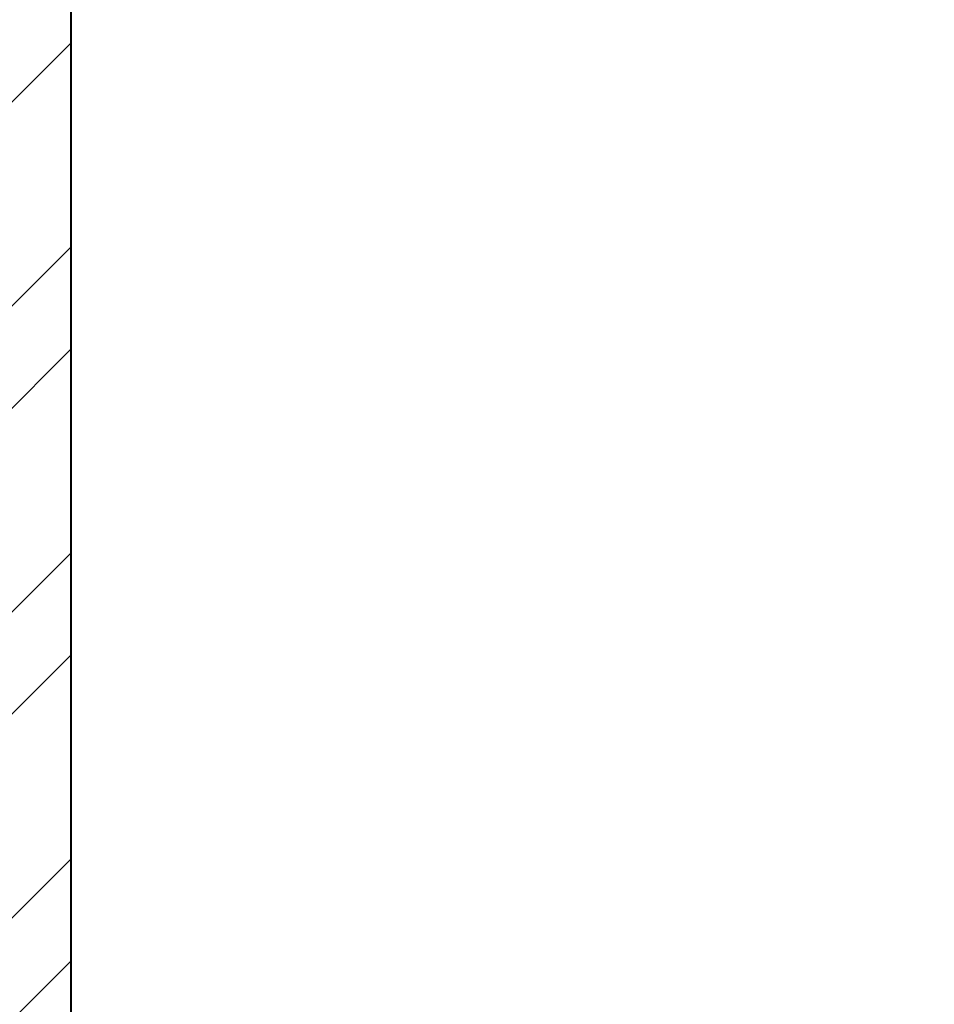
# Model space of a CAD drawing. Units: inches. Extents: x 2063 to 2617, y 1299 to 2210.
# Tile 9 of 22: x 2202 to 2242, y 1901 to 1945. Entities that reach past the tile are written whole.
import ezdxf

# ---------------------------------------------------------------- set-up
doc = ezdxf.new("R2010")
doc.units = ezdxf.units.IN
doc.layers.add('A-WALL', color=7, linetype='Continuous', lineweight=40)
doc.layers.add('A-WALL-PATT', color=215, linetype='Continuous', lineweight=13, true_color=0xa953a0)

msp = doc.modelspace()

# ---------------------------------------------------------------- hatches: boundary and pattern name
at = {"layer": 'A-WALL-PATT'}
h = msp.add_hatch(dxfattribs=at)
h.set_pattern_fill('ANSI32', color=256)
h.paths.add_polyline_path([(2553.6442, 2128.8122), (2511.1703, 2128.8122), (2511.1703, 2124.3122), (2549.1442, 2124.3122), (2549.1442, 2095.662), (2553.6442, 2095.662)])
h.paths.add_polyline_path([(2553.6442, 2035.662), (2549.1442, 2035.662), (2549.1442, 1980.3122), (2503.7214, 1980.3122), (2503.7214, 1975.8122), (2549.1442, 1975.8122), (2549.1442, 1962.9693), (2553.6442, 1962.9693)])
h.paths.add_polyline_path([(2553.6442, 1938.9693), (2549.1442, 1938.9693), (2549.1442, 1927.8122), (2477.1442, 1927.8122), (2477.1442, 1975.8122), (2481.2918, 1975.8122), (2481.2918, 1980.3122), (2453.2648, 1980.3122), (2453.2648, 1975.8122), (2472.6442, 1975.8122), (2472.6442, 1868.3122), (2400.6442, 1868.3122), (2400.6442, 1861.3782), (2405.1442, 1861.3782), (2405.1442, 1863.8122), (2480.9699, 1863.8122), (2480.9699, 1866.0622), (2480.9699, 1868.3122), (2477.1442, 1868.3122), (2477.1442, 1923.3122), (2549.1442, 1923.3122), (2549.1442, 1908.8504), (2553.6442, 1908.8504)])
h.paths.add_polyline_path([(2553.6442, 1884.8504), (2549.1442, 1884.8504), (2549.1442, 1868.3122), (2501.0636, 1868.3122), (2501.0636, 1863.8122), (2549.1442, 1863.8122), (2549.1442, 1826.0298), (2553.6442, 1826.0298)])
h.paths.add_polyline_path([(2388.1504, 1980.3122), (2340.6442, 1980.3122), (2340.6442, 2124.3122), (2358.7501, 2124.3122), (2358.7501, 2128.8122), (2316.3482, 2128.8122), (2316.3482, 2124.3122), (2336.1442, 2124.3122), (2336.1442, 1980.3122), (2289.1737, 1980.3122), (2289.1737, 1975.8122), (2336.1442, 1975.8122), (2336.1442, 1619.3122), (2333.1433, 1619.3122), (2333.1433, 1614.8122), (2344.1671, 1614.8122), (2344.1671, 1617.0622), (2344.1671, 1619.3122), (2340.6442, 1619.3122), (2340.6442, 1975.8122), (2388.1504, 1975.8122), (2388.1504, 1978.0622)])
h.paths.add_polyline_path([(2290.1442, 1614.8122), (2301.4594, 1614.8122), (2301.4594, 1617.0622), (2301.4594, 1619.3122), (2285.6442, 1619.3122), (2285.6442, 1566.8122), (2280.8619, 1566.8122), (2280.8619, 1564.5622), (2280.8619, 1562.3122), (2285.6442, 1562.3122), (2285.6442, 1442.3122), (2281.7879, 1442.3122), (2281.7879, 1437.8122), (2285.6442, 1437.8122), (2285.6442, 1401.8122), (2290.1442, 1401.8122)])
h.paths.add_polyline_path([(2549.1442, 1731.8122), (2405.1442, 1731.8122), (2405.1442, 1834.4638), (2402.8942, 1834.4638), (2400.6442, 1834.4638), (2400.6442, 1727.3122), (2549.1442, 1727.3122)])
h.paths.add_polyline_path([(2553.6442, 1766.0298), (2551.3942, 1766.0298), (2549.1442, 1766.0298), (2549.1442, 1686.7767), (2553.6442, 1686.7767)])
h.paths.add_polyline_path([(2553.6442, 1638.7767), (2551.3942, 1638.7767), (2549.1442, 1638.7767), (2549.1442, 1619.3122), (2448.6442, 1619.3122), (2448.6442, 1610.5671), (2450.8942, 1610.5671), (2453.1442, 1610.5671), (2453.1442, 1614.8122), (2549.1442, 1614.8122), (2549.1442, 1601.6421), (2553.6442, 1601.6421)])
h.paths.add_polyline_path([(2553.6442, 1577.6421), (2551.3942, 1577.6421), (2549.1442, 1577.6421), (2549.1442, 1566.8122), (2453.1442, 1566.8122), (2453.1442, 1591.5045), (2451.0335, 1591.5045), (2448.6442, 1591.5045), (2448.6442, 1566.8122), (2434.0475, 1566.8122), (2434.0475, 1562.3122), (2549.1442, 1562.3122), (2549.1442, 1533.48), (2553.6442, 1533.48)])
h.paths.add_polyline_path([(2553.6442, 1473.48), (2549.1442, 1473.48), (2549.1442, 1442.3122), (2502.6258, 1442.3122), (2502.6258, 1437.8122), (2549.1442, 1437.8122), (2549.1442, 1401.8122), (2553.6442, 1401.8122)])
h.paths.add_polyline_path([(2395.6442, 1562.3122), (2400.0901, 1562.3122), (2400.0901, 1564.5622), (2400.0901, 1566.8122), (2395.6442, 1566.8122), (2395.6442, 1619.3122), (2379.1127, 1619.3122), (2379.1127, 1614.8122), (2391.1442, 1614.8122), (2391.1442, 1401.8122), (2395.6442, 1401.8122), (2395.6442, 1437.8122), (2399.2425, 1437.8122), (2399.2425, 1440.0622), (2399.2425, 1442.3122), (2395.6442, 1442.3122)])
h.paths.add_polyline_path([(2442.6258, 1442.3122), (2419.6262, 1442.3122), (2419.6262, 1437.8122), (2442.6258, 1437.8122), (2442.6258, 1440.0622)])
h.paths.add_polyline_path([(2127.6442, 1480.2532), (2125.3942, 1480.2532), (2123.1442, 1480.2532), (2123.1442, 1401.8122), (2127.6442, 1401.8122), (2127.6442, 1437.8122), (2145.1538, 1437.8122), (2145.1538, 1440.0622), (2145.1538, 1442.3122), (2127.6442, 1442.3122)])
h.paths.add_polyline_path([(2259.809, 1442.3122), (2205.1538, 1442.3122), (2205.1538, 1437.8122), (2259.809, 1437.8122), (2259.809, 1440.0622)])
h.paths.add_polyline_path([(2127.6442, 1659.7652), (2123.1442, 1659.7652), (2123.1442, 1605.5161), (2125.3942, 1605.5161), (2127.6442, 1605.5161), (2127.6442, 1614.8122), (2223.6442, 1614.8122), (2223.6442, 1611.2723), (2228.1442, 1611.2723), (2228.1442, 1619.3122), (2127.6442, 1619.3122)])
h.paths.add_polyline_path([(2244.8673, 1566.8122), (2228.1442, 1566.8122), (2228.1442, 1590.8122), (2225.8942, 1590.8122), (2223.6442, 1590.8122), (2223.6442, 1566.8122), (2127.6442, 1566.8122), (2127.6442, 1581.5161), (2123.1442, 1581.5161), (2123.1442, 1540.2532), (2127.6442, 1540.2532), (2127.6442, 1562.3122), (2244.8673, 1562.3122), (2244.8673, 1564.5622)])
h.paths.add_polyline_path([(2172.5174, 1868.3122), (2127.6442, 1868.3122), (2127.6442, 1886.5833), (2123.1442, 1886.5833), (2123.1442, 1832.6633), (2127.6442, 1832.6633), (2127.6442, 1863.8122), (2172.5174, 1863.8122), (2172.5174, 1866.0622)])
h.paths.add_polyline_path([(2276.1442, 1868.3122), (2204.1442, 1868.3122), (2204.1442, 1923.3122), (2204.1442, 1975.8122), (2224.8362, 1975.8122), (2224.8362, 1978.1097), (2224.8362, 1980.3122), (2195.0729, 1980.3122), (2195.0729, 1978.0622), (2195.0729, 1975.8122), (2199.6442, 1975.8122), (2199.6442, 1927.8122), (2127.6442, 1927.8122), (2127.6442, 1942.3492), (2123.1442, 1942.3492), (2123.1442, 1910.5833), (2127.6442, 1910.5833), (2127.6442, 1923.3122), (2199.6442, 1923.3122), (2199.6442, 1868.3122), (2194.8228, 1868.3122), (2194.8228, 1864.7337), (2194.8228, 1863.8122), (2271.6442, 1863.8122), (2271.6442, 1860.0507), (2276.1442, 1860.0507)])
h.paths.add_polyline_path([(2276.1442, 1829.994), (2273.8942, 1829.994), (2271.6442, 1829.994), (2271.6442, 1731.8122), (2127.6442, 1731.8122), (2127.6442, 1772.6633), (2123.1442, 1772.6633), (2123.1442, 1707.7652), (2127.6442, 1707.7652), (2127.6442, 1727.3122), (2276.1442, 1727.3122)])
h.paths.add_polyline_path([(2127.6442, 2022.1152), (2123.1442, 2022.1152), (2123.1442, 1966.3492), (2127.6442, 1966.3492), (2127.6442, 1975.8122), (2174.2082, 1975.8122), (2174.2082, 1978.0622), (2174.2082, 1980.3122), (2127.6442, 1980.3122)])
h.paths.add_polyline_path([(2361.9755, 1678.588), (2398.4558, 1678.588), (2398.4558, 1697.2453), (2361.9755, 1697.2453)], flags=9)
h.paths.add_polyline_path([(2351.5397, 1780.4072), (2386.1987, 1780.4072), (2386.1987, 1790.7107), (2351.5397, 1790.7107)], flags=25)
h.paths.add_polyline_path([(2350.6753, 1940.9321), (2387.6024, 1940.9321), (2387.6024, 1959.5894), (2350.6753, 1959.5894)], flags=25)
h.paths.add_polyline_path([(2254.9545, 1684.638), (2295.0943, 1684.638), (2295.0943, 1703.2953), (2254.9545, 1703.2953)], flags=9)
h.paths.add_polyline_path([(2282.4946, 1782.4438), (2317.1535, 1782.4438), (2317.1535, 1792.7474), (2282.4946, 1792.7474)], flags=9)
h.paths.add_polyline_path([(2270.327, 1939.2854), (2307.254, 1939.2854), (2307.254, 1957.9428), (2270.327, 1957.9428)], flags=9)

# ---------------------------------------------------------------- linework, layer by layer
at = {"layer": 'A-WALL'}
for p, q in [((2204.1442, 1975.8122), (2204.1442, 1923.3122)), ((2204.1442, 1923.3122), (2204.1442, 1868.3122))]:
    msp.add_line(p, q, dxfattribs=at)

doc.saveas('drawing.dxf')
